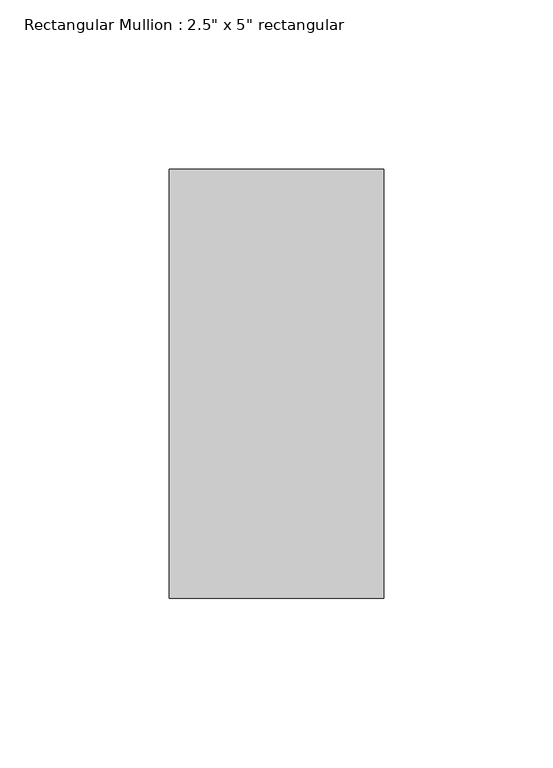
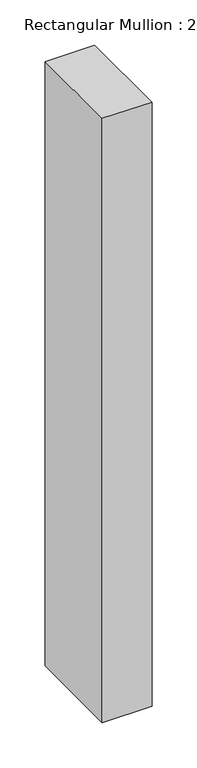
"""IFC4 building model written with IfcOpenShell, lengths in millimetres: member geometry."""

from ifc_helpers import new_model, si_unit, frame, origin, place, context, project, spatial, polyline, outline, extrude, source, transform, mapped, element, save


def member_2e6d4a6b(model_context):
    return source(origin(), model_context, "Body", "SweptSolid", [
        extrude(outline(polyline([(0.0, 63.5), (0.0, -63.5), (-63.5, -63.5), (-63.5, 63.5), (0.0, 63.5)])), frame((0.0, 0.0, -817.650384), z_axis=(0.0, 0.0, 1.0), x_axis=(1.0, 0.0, 0.0)), (0.0, 0.0, 1.0), 817.650384),
    ])


if __name__ == "__main__":
    model = new_model("IFC4")
    model_context = context("Model", 3, world=origin())
    ifc_project = project(units=[si_unit("LENGTHUNIT", "METRE", prefix="MILLI")], contexts=[model_context])
    site = spatial("IfcSite", under=ifc_project)
    building = spatial("IfcBuilding", under=site)
    placement = place(None, origin())
    member_shape = member_2e6d4a6b(model_context)
    element("IfcMember", 1, ObjectType="Rectangular Mullion : 2.5\" x 5\" rectangular", at=placement, inside=building, context=model_context, shape_type="MappedRepresentation", body=[
        mapped(member_shape, transform((0.0, 0.0, 0.0), x_axis=(1.0, 0.0, 0.0), y_axis=(0.0, 1.0, 0.0), z_axis=(0.0, 0.0, 1.0))),
    ])
    save(model, "model.ifc")

# Revit data of these elements
# Type "Rectangular Mullion : 2.5\" x 5\" rectangular"
#   built-in parameter 1007304 = 0.416667 (stored number, unit not read)
#   built-in parameter 1007301 = 0.104167 (stored number, unit not read)
#   built-in parameter 1007300 = 0.104167 (stored number, unit not read)
# Element 1 (IfcMember, "Rectangular Mullion : 2.5\" x 5\" rectangular")
#   Materials on its faces: "Aluminum"
# Materials
#   "Aluminum": class "Metal", colour RGB 247 247 247, transparency 0, Description = "Aluminum 6061", Cost = 0
